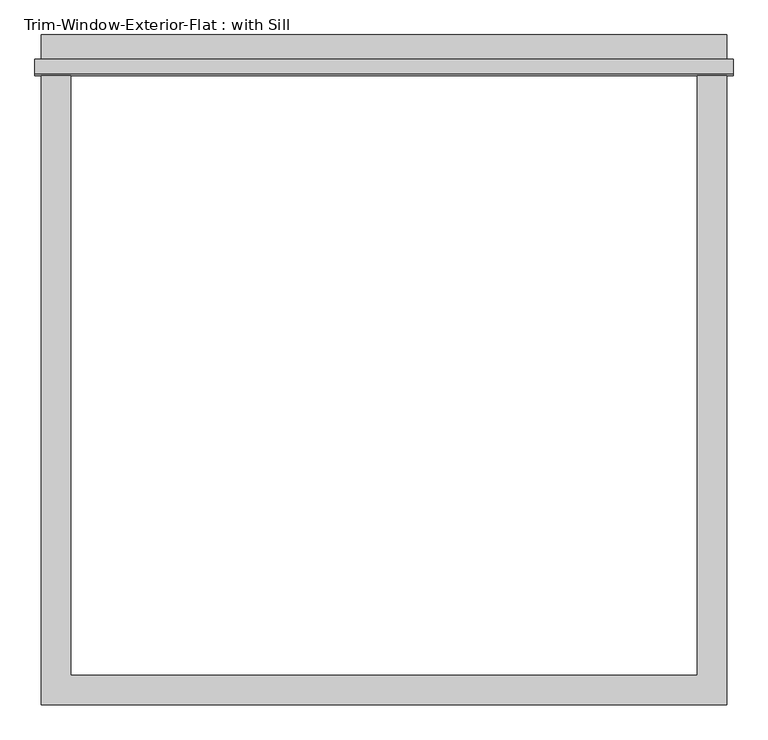
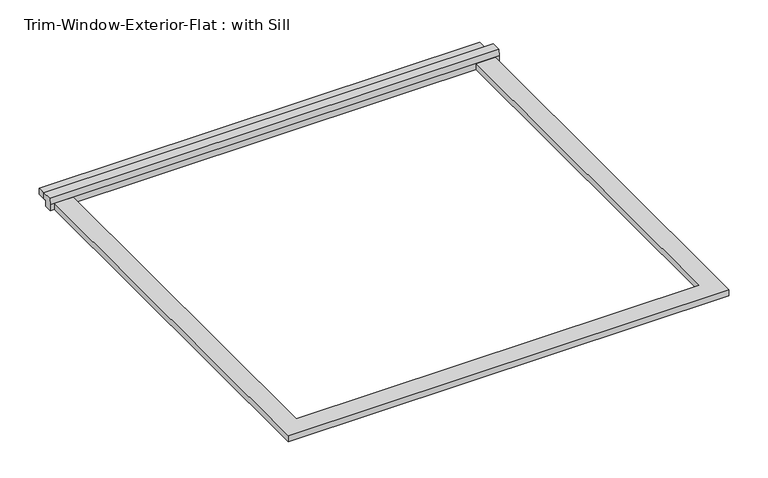
"""IFC4 building model written with IfcOpenShell, lengths in millimetres: proxy geometry, Trim-Window-Exterior-Flat : with Sill."""

from ifc_helpers import new_model, si_unit, frame, origin, origin_with_axes, place, context, project, spatial, polyline, outline, extrude, source, transform, mapped, element, save


def trim_window_exterior_flat_with_sill_c7d07f6c(model_context):
    return source(origin(), model_context, "Body", "SweptSolid", [
        extrude(outline(polyline([(666.75, 1190.5823709), (-666.75, 1190.5823709), (-666.75, 1247.7323709), (666.75, 1247.7323709), (666.75, 1190.5823709)])), origin_with_axes(), (0.0, 0.0, 1.0), 19.05),
        extrude(outline(polyline([(1200.15, 38.1), (1200.15, 19.05), (1190.5823709, 19.05), (1190.5823709, 0.0), (1168.4, 0.0), (1168.4, 19.05), (1170.8580645, 38.1), (1200.15, 38.1)])), frame((-679.45, 0.0, 0.0), z_axis=(1.0, 0.0, 0.0), x_axis=(0.0, 1.0, 0.0)), (0.0, 0.0, 1.0), 1358.9),
        extrude(outline(polyline([(-666.75, -57.15), (-666.75, 1168.4), (-609.6, 1168.4), (-609.6, 0.0), (609.6, 0.0), (609.6, 1168.4), (666.75, 1168.4), (666.75, -57.15), (-666.75, -57.15)])), origin_with_axes(), (0.0, 0.0, 1.0), 19.05),
    ])


if __name__ == "__main__":
    model = new_model("IFC4")
    model_context = context("Model", 3, world=origin())
    ifc_project = project(units=[si_unit("LENGTHUNIT", "METRE", prefix="MILLI")], contexts=[model_context])
    site = spatial("IfcSite", under=ifc_project)
    building = spatial("IfcBuilding", under=site)
    placement = place(None, origin())
    trim_window_exterior_flat_with_sill_shape = trim_window_exterior_flat_with_sill_c7d07f6c(model_context)
    element("IfcBuildingElementProxy", 1, Name="Trim-Window-Exterior-Flat : with Sill", ObjectType="Trim-Window-Exterior-Flat : with Sill", at=placement, inside=building, context=model_context, shape_type="MappedRepresentation", body=[
        mapped(trim_window_exterior_flat_with_sill_shape, transform((0.0, 0.0, 0.0), x_axis=(1.0, 0.0, 0.0), y_axis=(0.0, 1.0, 0.0), z_axis=(0.0, 0.0, 1.0))),
    ])
    save(model, "model.ifc")

# Revit data of these elements
# Type "Trim-Window-Exterior-Flat : with Sill"
#   Trim Width = 0' - 2 1/4"
#   Trim Thickness_Picture Frame = 0' - 1 1/4"
#   Trim Thickness_with Sill = 0' - 0 3/4"
#   Sill Thickness = 0' - 1 1/4"
#   Opening Width [instance default] = 2' - 0"
#   Opening Height [instance default] = 3' - 0"
#   Default Elevation = 4' - 0"
#   Sill = yes
#   Picture Frame = no
#   Trim Material [instance default] = none
# Element 1 (IfcBuildingElementProxy, "Trim-Window-Exterior-Flat : with Sill")
#   Opening Width = 4' - 0"
#   Opening Height = 3' - 10"
#   Trim Material = Clad - White
#   Materials on its faces: "Clad - White"
# Materials
#   "Clad - White": class "Wood", colour RGB 242 242 238, transparency 0, Cost = 0
